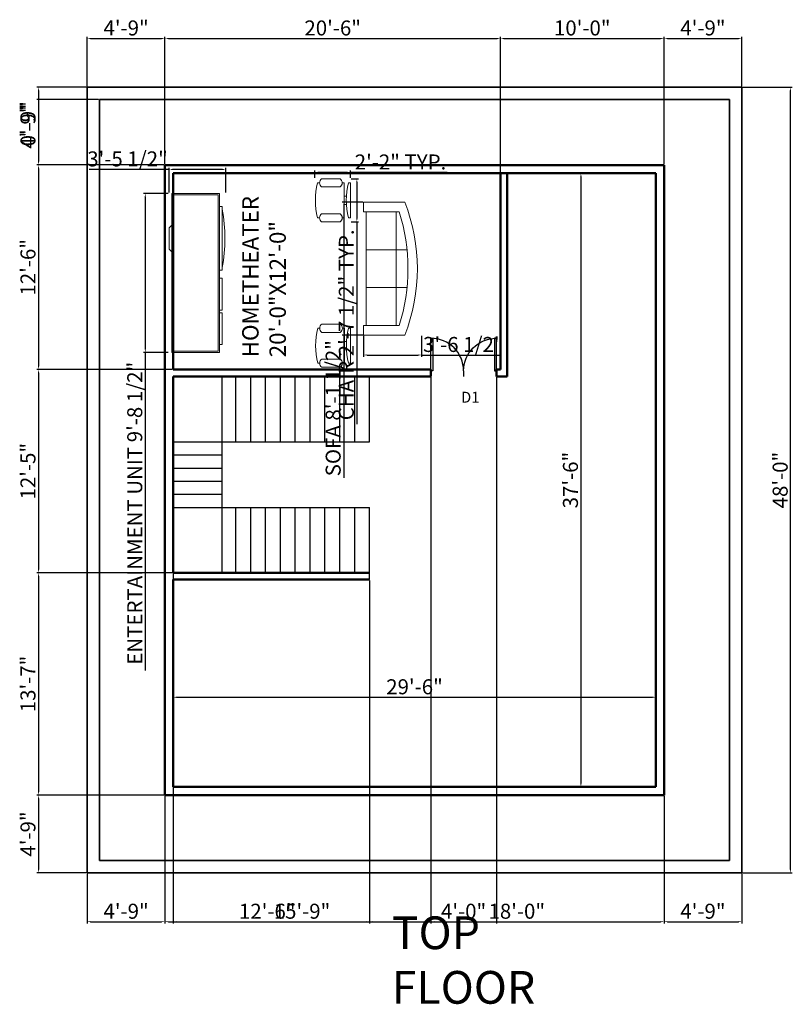
# Model space of a CAD drawing. Units: inches. Extents: x 2299 to 4423, y 1066 to 1805.
# Tile 7 of 7: x 3856 to 4423, y 1075 to 1796. Entities that reach past the tile are written whole.
import ezdxf

# ---------------------------------------------------------------- set-up
doc = ezdxf.new("R2010")
doc.units = ezdxf.units.IN
for name, color, linetype, lineweight in [('A-ANNO-DIMS', 2, 'Continuous', 18), ('A-ANNO-TEXT', 1, 'Continuous', 25), ('A-AREA-IDEN', 1, 'Continuous', 25), ('A-DOOR', 5, 'Continuous', 25), ('A-FLOR-STRS', 6, 'Continuous', 25), ('A-FURN', 8, 'Continuous', 18), ('A-WALL', 7, 'Continuous', 50), ('C-PROP', 7, 'Continuous', 35)]:
    doc.layers.add(name, color=color, linetype=linetype, lineweight=lineweight)
doc.styles.get("Standard").update_dxf_attribs({"font": 'arial.ttf'})
doc.dimstyles.new('ISO-25', dxfattribs={"dimtxt": 11, "dimasz": 2.5, "dimexe": 1.25, "dimexo": 0.625, "dimtad": 1, "dimlunit": 4, "dimtxsty": 'Standard', "dimcen": 2.5, "dimadec": 0, "dimazin": 0, "dimtfac": 1, "dimtmove": 0, "dimatfit": 3, "dimfxl": 1, "dimarcsym": 0})

# ---------------------------------------------------------------- blocks, each defined once
blk = doc.blocks.new('*U2')
for p, q in [((0, 0), (0, -5)), ((30, 0), (30, -5))]:
    blk.add_line(p, q)
blk.add_lwpolyline([(0, 0), (0, 30), (1.75, 30), (1.75, 0)], close=True)
blk.add_arc((0, 0), 30, 0, 90)
blk = doc.blocks.new('Entertainment Center')
for p, q in [((-4, 0), (-5, -1)), ((4, 0), (-4, 0)), ((5, -1), (4, 0)), ((-17, -19), (-17, -1)), ((-17, -1), (43, -1)), ((-16.5, -18.5), (-16.5, -1.5)), ((-16.5, -1.5), (42.5, -1.5)), ((42.5, -1.5), (42.5, -18.5)), ((43, -1), (43, -19)), ((42.5, -18.5), (-16.5, -18.5)), ((43, -19), (-17, -19)), ((-12, -20), (-12, -19)), ((12, -20), (-12, -20)), ((12, -19), (12, -20)), ((15, -20), (15, -19)), ((27, -20), (15, -20)), ((27, -19), (27, -20)), ((28, -20), (28, -19)), ((40, -20), (28, -20)), ((40, -19), (40, -20))]:
    blk.add_line(p, q)
blk.add_arc((0, 40), 61, 259.6111, 280.3889)
blk = doc.blocks.new('Sofa - Roundback 7 ft.')
for p, q in [((-36.000027, -34), (-36.000027, -11.4696)), ((-12.00002, -32.4421), (-12.00003, -6.5971)), ((11.99997, -32.4421), (11.99998, -6.5971)), ((35.99998, -34), (35.99998, -11.4696)), ((-35.999844, -13.3819), (35.9998, -13.3819)), ((-36.000027, -32.4421), (35.99998, -32.4421))]:
    blk.add_line(p, q)
for points in [[(-36.000027, -34), (-42.000027, -34), (-42.000027, -8)], [(41.99998, -8), (41.99998, -34), (35.99998, -34)]]:
    blk.add_lwpolyline(points)
for centre, radius, start, end in [((0, -114.25), 114.25, 68.43141, 111.5686), ((-0.00001, -127.1968), 121.1968, 72.72033, 107.2797)]:
    blk.add_arc(centre, radius, start, end)
blk = doc.blocks.new('Chair - Desk')
for p, q in [((-8.5, 0), (-8.5, -1)), ((-8.5, 0), (8.5, 0)), ((8.5, 0), (8.5, -1)), ((-8.5, -3), (-8.5, -4)), ((-8.5, -3), (8.5, -3)), ((-2, -3), (-2, -1.9355)), ((2, -1.9576), (2, -3)), ((8.5, -3), (8.5, -4)), ((-10.5, -5), (-10.5, -14)), ((-6.5, -14), (-6.5, -5)), ((6.5, -5), (6.5, -14)), ((10.5, -14), (10.5, -5)), ((-8.5, -15), (-8.5, -16)), ((8.5, -15), (8.5, -16))]:
    blk.add_line(p, q)
for centre, radius, start, end in [((-8.5, -6.5), 2.5, 36.8699, 143.1301), ((0, 34.625), 36.625, 256.5803, 283.4197), ((8.5, -6.5), 2.5, 36.8699, 143.1301), ((-8.5, -12.5), 2.5, 216.8699, 323.1301), ((8.5, -12.5), 2.5, 216.8699, 323.1301), ((0, 19.625), 36.625, 256.5803, 283.4197)]:
    blk.add_arc(centre, radius, start, end)
blk = doc.blocks.new('*D28')
at = {"layer": 'A-ANNO-DIMS', "color": 0, "lineweight": -2, "transparency": 16777216}
for p, q in [((3969.03, 1234.57), (3969.03, 1300.97)), ((3971.53, 1299.72), (4320.53, 1299.72)), ((4323.03, 1234.57), (4323.03, 1300.97))]:
    blk.add_line(p, q, dxfattribs=at)
at = {"layer": 'A-ANNO-DIMS', "color": 0, "transparency": 16777216}
for points in [[(3971.53, 1300.14), (3971.53, 1299.31), (3969.03, 1299.72)], [(4320.53, 1300.14), (4320.53, 1299.31), (4323.03, 1299.72)]]:
    blk.add_solid(points, dxfattribs=at)
at = {"layer": 'Defpoints', "color": 0, "transparency": 16777216}
for p in [(4323.03, 1299.72), (3969.03, 1233.95), (4323.03, 1233.95)]:
    blk.add_point(p, dxfattribs=at)
at = {"layer": 'A-ANNO-DIMS', "color": 0, "transparency": 16777216, "insert": (4146.03, 1305.96), "char_height": 11, "attachment_point": 5}
blk.add_mtext('29\'-6"', dxfattribs=at)
blk = doc.blocks.new('*D29')
at = {"layer": 'A-ANNO-DIMS', "color": 0, "lineweight": -2, "transparency": 16777216}
for p, q in [((4322.4, 1683.95), (4266.78, 1683.95)), ((4268.03, 1681.45), (4268.03, 1236.45)), ((4322.4, 1233.95), (4266.78, 1233.95))]:
    blk.add_line(p, q, dxfattribs=at)
at = {"layer": 'A-ANNO-DIMS', "color": 0, "transparency": 16777216}
for points in [[(4267.62, 1681.45), (4268.45, 1681.45), (4268.03, 1683.95)], [(4267.62, 1236.45), (4268.45, 1236.45), (4268.03, 1233.95)]]:
    blk.add_solid(points, dxfattribs=at)
at = {"layer": 'Defpoints', "color": 0, "transparency": 16777216}
for p in [(4323.03, 1683.95), (4268.03, 1233.95), (4323.03, 1233.95)]:
    blk.add_point(p, dxfattribs=at)
at = {"layer": 'A-ANNO-DIMS', "color": 0, "transparency": 16777216, "insert": (4261.79, 1458.95), "char_height": 11, "attachment_point": 5, "rotation": 90}
blk.add_mtext('37\'-6"', dxfattribs=at)
blk = doc.blocks.new('*D36')
at = {"layer": 'A-ANNO-DIMS', "color": 0, "lineweight": -2, "transparency": 16777216}
for p, q in [((4099.63, 1679.84), (4105, 1679.84)), ((4103.75, 1677.34), (4103.75, 1650.71)), ((4099.63, 1648.21), (4105, 1648.21)), ((4103.75, 1648.21), (4103.75, 1499.82))]:
    blk.add_line(p, q, dxfattribs=at)
at = {"layer": 'A-ANNO-DIMS', "color": 0, "transparency": 16777216}
for points in [[(4103.33, 1677.34), (4104.16, 1677.34), (4103.75, 1679.84)], [(4103.33, 1650.71), (4104.16, 1650.71), (4103.75, 1648.21)]]:
    blk.add_solid(points, dxfattribs=at)
at = {"layer": 'Defpoints', "color": 0, "transparency": 16777216}
for p in [(4099, 1679.84), (4099, 1648.21), (4103.75, 1648.21)]:
    blk.add_point(p, dxfattribs=at)
at = {"layer": 'A-ANNO-DIMS', "color": 0, "transparency": 16777216, "insert": (4097.44, 1572.76), "char_height": 11, "attachment_point": 5, "rotation": 90}
blk.add_mtext('CHAIR 2\'-7 1/2" TYP.', dxfattribs=at)
blk = doc.blocks.new('*D37')
at = {"layer": 'A-ANNO-DIMS', "color": 0, "lineweight": -2, "transparency": 16777216}
for p, q in [((4072.89, 1680.47), (4072.89, 1685.84)), ((4075.39, 1684.59), (4096.5, 1684.59)), ((4099, 1680.47), (4099, 1685.84)), ((4099, 1684.59), (4169.99, 1684.59))]:
    blk.add_line(p, q, dxfattribs=at)
at = {"layer": 'A-ANNO-DIMS', "color": 0, "transparency": 16777216}
for points in [[(4075.39, 1685), (4075.39, 1684.17), (4072.89, 1684.59)], [(4096.5, 1685), (4096.5, 1684.17), (4099, 1684.59)]]:
    blk.add_solid(points, dxfattribs=at)
at = {"layer": 'Defpoints', "color": 0, "transparency": 16777216}
for p in [(4099, 1684.59), (4072.89, 1679.84), (4099, 1679.84)]:
    blk.add_point(p, dxfattribs=at)
at = {"layer": 'A-ANNO-DIMS', "color": 0, "transparency": 16777216, "insert": (4135.75, 1690.74), "char_height": 11, "attachment_point": 5}
blk.add_mtext('2\'-2" TYP.', dxfattribs=at)
blk = doc.blocks.new('*D42')
at = {"layer": 'A-ANNO-DIMS', "color": 0, "lineweight": -2, "transparency": 16777216}
for p, q in [((3965.48, 1669.16), (3947.35, 1669.16)), ((3948.6, 1666.66), (3948.6, 1554.92)), ((3965.48, 1552.42), (3947.35, 1552.42)), ((3948.6, 1552.42), (3948.6, 1319.37))]:
    blk.add_line(p, q, dxfattribs=at)
at = {"layer": 'A-ANNO-DIMS', "color": 0, "transparency": 16777216}
for points in [[(3948.18, 1666.66), (3949.01, 1666.66), (3948.6, 1669.16)], [(3948.18, 1554.92), (3949.01, 1554.92), (3948.6, 1552.42)]]:
    blk.add_solid(points, dxfattribs=at)
at = {"layer": 'Defpoints', "color": 0, "transparency": 16777216}
for p in [(3966.11, 1669.16), (3948.6, 1552.42), (3966.11, 1552.42)]:
    blk.add_point(p, dxfattribs=at)
at = {"layer": 'A-ANNO-DIMS', "color": 0, "transparency": 16777216, "insert": (3942.29, 1434.64), "char_height": 11, "attachment_point": 5, "rotation": 90}
blk.add_mtext('ENTERTAINMENT UNIT 9\'-8 1/2"', dxfattribs=at)
blk = doc.blocks.new('*D43')
at = {"layer": 'A-ANNO-DIMS', "color": 0, "lineweight": -2, "transparency": 16777216}
for p, q in [((3966.11, 1686.67), (3907.49, 1686.67)), ((3966.11, 1669.79), (3966.11, 1687.92)), ((4005.12, 1686.67), (3968.61, 1686.67)), ((4007.62, 1669.79), (4007.62, 1687.92))]:
    blk.add_line(p, q, dxfattribs=at)
at = {"layer": 'A-ANNO-DIMS', "color": 0, "transparency": 16777216}
for points in [[(3968.61, 1687.09), (3968.61, 1686.25), (3966.11, 1686.67)], [(4005.12, 1687.09), (4005.12, 1686.25), (4007.62, 1686.67)]]:
    blk.add_solid(points, dxfattribs=at)
at = {"layer": 'Defpoints', "color": 0, "transparency": 16777216}
for p in [(3966.11, 1686.67), (3966.11, 1669.16), (4007.62, 1669.16)]:
    blk.add_point(p, dxfattribs=at)
at = {"layer": 'A-ANNO-DIMS', "color": 0, "transparency": 16777216, "insert": (3935.55, 1692.99), "char_height": 11, "attachment_point": 5}
blk.add_mtext('3\'-5 1/2"', dxfattribs=at)
blk = doc.blocks.new('*D54')
at = {"layer": 'A-ANNO-DIMS', "color": 0, "lineweight": -2, "transparency": 16777216}
for p, q in [((4108.1, 1662.66), (4092.86, 1662.66)), ((4094.11, 1660.16), (4094.11, 1567.74)), ((4108.1, 1565.24), (4092.86, 1565.24)), ((4094.11, 1565.24), (4094.11, 1460.56))]:
    blk.add_line(p, q, dxfattribs=at)
at = {"layer": 'A-ANNO-DIMS', "color": 0, "transparency": 16777216}
for points in [[(4093.7, 1660.16), (4094.53, 1660.16), (4094.11, 1662.66)], [(4093.7, 1567.74), (4094.53, 1567.74), (4094.11, 1565.24)]]:
    blk.add_solid(points, dxfattribs=at)
at = {"layer": 'Defpoints', "color": 0, "transparency": 16777216}
for p in [(4108.73, 1662.66), (4094.11, 1565.24), (4108.73, 1565.24)]:
    blk.add_point(p, dxfattribs=at)
at = {"layer": 'A-ANNO-DIMS', "color": 0, "transparency": 16777216, "insert": (4087.8, 1511.65), "char_height": 11, "attachment_point": 5, "rotation": 90}
blk.add_mtext('SOFA 8\'-1 1/2"', dxfattribs=at)
blk = doc.blocks.new('*D55')
at = {"layer": 'A-ANNO-DIMS', "color": 0, "lineweight": -2, "transparency": 16777216}
for p, q in [((4108.73, 1564.61), (4108.73, 1549.38)), ((4151.25, 1564.61), (4151.25, 1549.38)), ((4111.23, 1550.63), (4148.75, 1550.63)), ((4151.25, 1550.63), (4209.87, 1550.63))]:
    blk.add_line(p, q, dxfattribs=at)
at = {"layer": 'A-ANNO-DIMS', "color": 0, "transparency": 16777216}
for points in [[(4111.23, 1551.04), (4111.23, 1550.21), (4108.73, 1550.63)], [(4148.75, 1551.04), (4148.75, 1550.21), (4151.25, 1550.63)]]:
    blk.add_solid(points, dxfattribs=at)
at = {"layer": 'Defpoints', "color": 0, "transparency": 16777216}
for p in [(4108.73, 1565.24), (4151.25, 1565.24), (4151.25, 1550.63)]:
    blk.add_point(p, dxfattribs=at)
at = {"layer": 'A-ANNO-DIMS', "color": 0, "transparency": 16777216, "insert": (4181.81, 1556.94), "char_height": 11, "attachment_point": 5}
blk.add_mtext('3\'-6 1/2"', dxfattribs=at)
blk = doc.blocks.new('*D115')
at = {"layer": 'A-ANNO-DIMS', "color": 0, "lineweight": -2, "transparency": 16777216}
for p, q in [((3906.03, 1747.57), (3906.03, 1784)), ((3963.03, 1690.57), (3963.03, 1784)), ((3908.53, 1782.75), (3960.53, 1782.75))]:
    blk.add_line(p, q, dxfattribs=at)
at = {"layer": 'A-ANNO-DIMS', "color": 0, "transparency": 16777216}
for points in [[(3908.53, 1783.16), (3908.53, 1782.33), (3906.03, 1782.75)], [(3960.53, 1783.16), (3960.53, 1782.33), (3963.03, 1782.75)]]:
    blk.add_solid(points, dxfattribs=at)
at = {"layer": 'Defpoints', "color": 0, "transparency": 16777216}
for p in [(3963.03, 1782.75), (3906.03, 1746.95), (3963.03, 1689.95)]:
    blk.add_point(p, dxfattribs=at)
at = {"layer": 'A-ANNO-DIMS', "color": 0, "transparency": 16777216, "insert": (3934.53, 1788.99), "char_height": 11, "attachment_point": 5}
blk.add_mtext('4\'-9"', dxfattribs=at)
blk = doc.blocks.new('*D116')
at = {"layer": 'A-ANNO-DIMS', "color": 0, "lineweight": -2, "transparency": 16777216}
for p, q in [((3963.03, 1690.57), (3963.03, 1784)), ((4209.03, 1684.57), (4209.03, 1784)), ((3965.53, 1782.75), (4206.53, 1782.75))]:
    blk.add_line(p, q, dxfattribs=at)
at = {"layer": 'A-ANNO-DIMS', "color": 0, "transparency": 16777216}
for points in [[(3965.53, 1783.16), (3965.53, 1782.33), (3963.03, 1782.75)], [(4206.53, 1783.16), (4206.53, 1782.33), (4209.03, 1782.75)]]:
    blk.add_solid(points, dxfattribs=at)
at = {"layer": 'Defpoints', "color": 0, "transparency": 16777216}
for p in [(4209.03, 1782.75), (3963.03, 1689.95), (4209.03, 1683.95)]:
    blk.add_point(p, dxfattribs=at)
at = {"layer": 'A-ANNO-DIMS', "color": 0, "transparency": 16777216, "insert": (4086.03, 1788.99), "char_height": 11, "attachment_point": 5}
blk.add_mtext('20\'-6"', dxfattribs=at)
blk = doc.blocks.new('*D117')
at = {"layer": 'A-ANNO-DIMS', "color": 0, "lineweight": -2, "transparency": 16777216}
for p, q in [((4209.03, 1684.57), (4209.03, 1784)), ((4329.03, 1690.57), (4329.03, 1784)), ((4211.53, 1782.75), (4326.53, 1782.75))]:
    blk.add_line(p, q, dxfattribs=at)
at = {"layer": 'A-ANNO-DIMS', "color": 0, "transparency": 16777216}
for points in [[(4211.53, 1783.16), (4211.53, 1782.33), (4209.03, 1782.75)], [(4326.53, 1783.16), (4326.53, 1782.33), (4329.03, 1782.75)]]:
    blk.add_solid(points, dxfattribs=at)
at = {"layer": 'Defpoints', "color": 0, "transparency": 16777216}
for p in [(4329.03, 1782.75), (4329.03, 1689.95), (4209.03, 1683.95)]:
    blk.add_point(p, dxfattribs=at)
at = {"layer": 'A-ANNO-DIMS', "color": 0, "transparency": 16777216, "insert": (4269.03, 1788.99), "char_height": 11, "attachment_point": 5}
blk.add_mtext('10\'-0"', dxfattribs=at)
blk = doc.blocks.new('*D118')
at = {"layer": 'A-ANNO-DIMS', "color": 0, "lineweight": -2, "transparency": 16777216}
for p, q in [((4329.03, 1690.57), (4329.03, 1784)), ((4386.03, 1747.57), (4386.03, 1784)), ((4331.53, 1782.75), (4383.53, 1782.75))]:
    blk.add_line(p, q, dxfattribs=at)
at = {"layer": 'A-ANNO-DIMS', "color": 0, "transparency": 16777216}
for points in [[(4331.53, 1783.16), (4331.53, 1782.33), (4329.03, 1782.75)], [(4383.53, 1783.16), (4383.53, 1782.33), (4386.03, 1782.75)]]:
    blk.add_solid(points, dxfattribs=at)
at = {"layer": 'Defpoints', "color": 0, "transparency": 16777216}
for p in [(4386.03, 1782.75), (4386.03, 1746.95), (4329.03, 1689.95)]:
    blk.add_point(p, dxfattribs=at)
at = {"layer": 'A-ANNO-DIMS', "color": 0, "transparency": 16777216, "insert": (4357.53, 1788.99), "char_height": 11, "attachment_point": 5}
blk.add_mtext('4\'-9"', dxfattribs=at)
blk = doc.blocks.new('*D119')
at = {"layer": 'A-ANNO-DIMS', "color": 0, "lineweight": -2, "transparency": 16777216}
for p, q in [((3905.4, 1746.95), (3868.98, 1746.95)), ((3870.23, 1744.45), (3870.23, 1692.45)), ((3962.4, 1689.95), (3868.98, 1689.95))]:
    blk.add_line(p, q, dxfattribs=at)
at = {"layer": 'A-ANNO-DIMS', "color": 0, "transparency": 16777216}
for points in [[(3869.81, 1744.45), (3870.64, 1744.45), (3870.23, 1746.95)], [(3869.81, 1692.45), (3870.64, 1692.45), (3870.23, 1689.95)]]:
    blk.add_solid(points, dxfattribs=at)
at = {"layer": 'Defpoints', "color": 0, "transparency": 16777216}
for p in [(3906.03, 1746.95), (3870.23, 1689.95), (3963.03, 1689.95)]:
    blk.add_point(p, dxfattribs=at)
at = {"layer": 'A-ANNO-DIMS', "color": 0, "transparency": 16777216, "insert": (3863.99, 1718.45), "char_height": 11, "attachment_point": 5, "rotation": 90}
blk.add_mtext('4\'-9"', dxfattribs=at)
blk = doc.blocks.new('*D120')
at = {"layer": 'A-ANNO-DIMS', "color": 0, "lineweight": -2, "transparency": 16777216}
for p, q in [((3962.4, 1689.95), (3868.98, 1689.95)), ((3870.23, 1687.45), (3870.23, 1542.45)), ((3968.4, 1539.95), (3868.98, 1539.95))]:
    blk.add_line(p, q, dxfattribs=at)
at = {"layer": 'A-ANNO-DIMS', "color": 0, "transparency": 16777216}
for points in [[(3869.81, 1687.45), (3870.64, 1687.45), (3870.23, 1689.95)], [(3869.81, 1542.45), (3870.64, 1542.45), (3870.23, 1539.95)]]:
    blk.add_solid(points, dxfattribs=at)
at = {"layer": 'Defpoints', "color": 0, "transparency": 16777216}
for p in [(3963.03, 1689.95), (3870.23, 1539.95), (3969.03, 1539.95)]:
    blk.add_point(p, dxfattribs=at)
at = {"layer": 'A-ANNO-DIMS', "color": 0, "transparency": 16777216, "insert": (3863.99, 1614.95), "char_height": 11, "attachment_point": 5, "rotation": 90}
blk.add_mtext('12\'-6"', dxfattribs=at)
blk = doc.blocks.new('*D121')
at = {"layer": 'A-ANNO-DIMS', "color": 0, "lineweight": -2, "transparency": 16777216}
for p, q in [((3968.4, 1539.95), (3868.98, 1539.95)), ((3870.23, 1537.45), (3870.23, 1393.45)), ((3968.4, 1390.95), (3868.98, 1390.95))]:
    blk.add_line(p, q, dxfattribs=at)
at = {"layer": 'A-ANNO-DIMS', "color": 0, "transparency": 16777216}
for points in [[(3869.81, 1537.45), (3870.64, 1537.45), (3870.23, 1539.95)], [(3869.81, 1393.45), (3870.64, 1393.45), (3870.23, 1390.95)]]:
    blk.add_solid(points, dxfattribs=at)
at = {"layer": 'Defpoints', "color": 0, "transparency": 16777216}
for p in [(3969.03, 1539.95), (3870.23, 1390.95), (3969.03, 1390.95)]:
    blk.add_point(p, dxfattribs=at)
at = {"layer": 'A-ANNO-DIMS', "color": 0, "transparency": 16777216, "insert": (3863.99, 1465.45), "char_height": 11, "attachment_point": 5, "rotation": 90}
blk.add_mtext('12\'-5"', dxfattribs=at)
blk = doc.blocks.new('*D122')
at = {"layer": 'A-ANNO-DIMS', "color": 0, "lineweight": -2, "transparency": 16777216}
for p, q in [((3968.4, 1390.95), (3868.98, 1390.95)), ((3870.23, 1388.45), (3870.23, 1230.45)), ((3962.4, 1227.95), (3868.98, 1227.95))]:
    blk.add_line(p, q, dxfattribs=at)
at = {"layer": 'A-ANNO-DIMS', "color": 0, "transparency": 16777216}
for points in [[(3869.81, 1388.45), (3870.64, 1388.45), (3870.23, 1390.95)], [(3869.81, 1230.45), (3870.64, 1230.45), (3870.23, 1227.95)]]:
    blk.add_solid(points, dxfattribs=at)
at = {"layer": 'Defpoints', "color": 0, "transparency": 16777216}
for p in [(3969.03, 1390.95), (3870.23, 1227.95), (3963.03, 1227.95)]:
    blk.add_point(p, dxfattribs=at)
at = {"layer": 'A-ANNO-DIMS', "color": 0, "transparency": 16777216, "insert": (3863.98, 1309.45), "char_height": 11, "attachment_point": 5, "rotation": 90}
blk.add_mtext('13\'-7"', dxfattribs=at)
blk = doc.blocks.new('*D123')
at = {"layer": 'A-ANNO-DIMS', "color": 0, "lineweight": -2, "transparency": 16777216}
for p, q in [((3962.4, 1227.95), (3868.98, 1227.95)), ((3870.23, 1225.45), (3870.23, 1173.45)), ((3905.4, 1170.95), (3868.98, 1170.95))]:
    blk.add_line(p, q, dxfattribs=at)
at = {"layer": 'A-ANNO-DIMS', "color": 0, "transparency": 16777216}
for points in [[(3869.81, 1225.45), (3870.64, 1225.45), (3870.23, 1227.95)], [(3869.81, 1173.45), (3870.64, 1173.45), (3870.23, 1170.95)]]:
    blk.add_solid(points, dxfattribs=at)
at = {"layer": 'Defpoints', "color": 0, "transparency": 16777216}
for p in [(3963.03, 1227.95), (3870.23, 1170.95), (3906.03, 1170.95)]:
    blk.add_point(p, dxfattribs=at)
at = {"layer": 'A-ANNO-DIMS', "color": 0, "transparency": 16777216, "insert": (3863.99, 1199.45), "char_height": 11, "attachment_point": 5, "rotation": 90}
blk.add_mtext('4\'-9"', dxfattribs=at)
blk = doc.blocks.new('*D124')
at = {"layer": 'A-ANNO-DIMS', "color": 0, "lineweight": -2, "transparency": 16777216}
for p, q in [((3905.4, 1746.95), (3868.98, 1746.95)), ((3870.23, 1744.45), (3870.23, 1740.45)), ((3914.4, 1737.95), (3868.98, 1737.95)), ((3870.23, 1737.95), (3870.23, 1704.95))]:
    blk.add_line(p, q, dxfattribs=at)
at = {"layer": 'A-ANNO-DIMS', "color": 0, "transparency": 16777216}
for points in [[(3869.81, 1744.45), (3870.64, 1744.45), (3870.23, 1746.95)], [(3869.81, 1740.45), (3870.64, 1740.45), (3870.23, 1737.95)]]:
    blk.add_solid(points, dxfattribs=at)
at = {"layer": 'Defpoints', "color": 0, "transparency": 16777216}
for p in [(3906.03, 1746.95), (3870.23, 1737.95), (3915.03, 1737.95)]:
    blk.add_point(p, dxfattribs=at)
at = {"layer": 'A-ANNO-DIMS', "color": 0, "transparency": 16777216, "insert": (3863.99, 1720.2), "char_height": 11, "attachment_point": 5, "rotation": 90}
blk.add_mtext('0\'-9"', dxfattribs=at)
blk = doc.blocks.new('*D125')
at = {"layer": 'A-ANNO-DIMS', "color": 0, "lineweight": -2, "transparency": 16777216}
for p, q in [((4386.65, 1746.95), (4423.08, 1746.95)), ((4421.83, 1173.45), (4421.83, 1744.45)), ((4386.65, 1170.95), (4423.08, 1170.95))]:
    blk.add_line(p, q, dxfattribs=at)
at = {"layer": 'A-ANNO-DIMS', "color": 0, "transparency": 16777216}
for points in [[(4421.41, 1744.45), (4422.24, 1744.45), (4421.83, 1746.95)], [(4421.41, 1173.45), (4422.24, 1173.45), (4421.83, 1170.95)]]:
    blk.add_solid(points, dxfattribs=at)
at = {"layer": 'Defpoints', "color": 0, "transparency": 16777216}
for p in [(4386.03, 1746.95), (4421.83, 1746.95), (4386.03, 1170.95)]:
    blk.add_point(p, dxfattribs=at)
at = {"layer": 'A-ANNO-DIMS', "color": 0, "transparency": 16777216, "insert": (4415.59, 1458.95), "char_height": 11, "attachment_point": 5, "rotation": 90}
blk.add_mtext('48\'-0"', dxfattribs=at)
blk = doc.blocks.new('*D126')
at = {"layer": 'A-ANNO-DIMS', "color": 0, "lineweight": -2, "transparency": 16777216}
for p, q in [((3963.03, 1227.32), (3963.03, 1133.9)), ((3906.03, 1170.32), (3906.03, 1133.9)), ((3908.53, 1135.15), (3960.53, 1135.15))]:
    blk.add_line(p, q, dxfattribs=at)
at = {"layer": 'A-ANNO-DIMS', "color": 0, "transparency": 16777216}
for points in [[(3908.53, 1135.56), (3908.53, 1134.73), (3906.03, 1135.15)], [(3960.53, 1135.56), (3960.53, 1134.73), (3963.03, 1135.15)]]:
    blk.add_solid(points, dxfattribs=at)
at = {"layer": 'Defpoints', "color": 0, "transparency": 16777216}
for p in [(3963.03, 1227.95), (3906.03, 1170.95), (3963.03, 1135.15)]:
    blk.add_point(p, dxfattribs=at)
at = {"layer": 'A-ANNO-DIMS', "color": 0, "transparency": 16777216, "insert": (3934.53, 1141.39), "char_height": 11, "attachment_point": 5}
blk.add_mtext('4\'-9"', dxfattribs=at)
blk = doc.blocks.new('*D127')
at = {"layer": 'A-ANNO-DIMS', "color": 0, "lineweight": -2, "transparency": 16777216}
for p, q in [((4113.03, 1385.32), (4113.03, 1133.9)), ((3963.03, 1227.32), (3963.03, 1133.9)), ((3965.53, 1135.15), (4110.53, 1135.15))]:
    blk.add_line(p, q, dxfattribs=at)
at = {"layer": 'A-ANNO-DIMS', "color": 0, "transparency": 16777216}
for points in [[(3965.53, 1135.56), (3965.53, 1134.73), (3963.03, 1135.15)], [(4110.53, 1135.56), (4110.53, 1134.73), (4113.03, 1135.15)]]:
    blk.add_solid(points, dxfattribs=at)
at = {"layer": 'Defpoints', "color": 0, "transparency": 16777216}
for p in [(4113.03, 1385.95), (3963.03, 1227.95), (4113.03, 1135.15)]:
    blk.add_point(p, dxfattribs=at)
at = {"layer": 'A-ANNO-DIMS', "color": 0, "transparency": 16777216, "insert": (4038.03, 1141.39), "char_height": 11, "attachment_point": 5}
blk.add_mtext('12\'-6"', dxfattribs=at)
blk = doc.blocks.new('*D128')
at = {"layer": 'A-ANNO-DIMS', "color": 0, "lineweight": -2, "transparency": 16777216}
for p, q in [((4113.03, 1385.32), (4113.03, 1133.9)), ((4329.03, 1227.32), (4329.03, 1133.9)), ((4115.53, 1135.15), (4326.53, 1135.15))]:
    blk.add_line(p, q, dxfattribs=at)
at = {"layer": 'A-ANNO-DIMS', "color": 0, "transparency": 16777216}
for points in [[(4115.53, 1135.56), (4115.53, 1134.73), (4113.03, 1135.15)], [(4326.53, 1135.56), (4326.53, 1134.73), (4329.03, 1135.15)]]:
    blk.add_solid(points, dxfattribs=at)
at = {"layer": 'Defpoints', "color": 0, "transparency": 16777216}
for p in [(4113.03, 1385.95), (4329.03, 1227.95), (4329.03, 1135.15)]:
    blk.add_point(p, dxfattribs=at)
at = {"layer": 'A-ANNO-DIMS', "color": 0, "transparency": 16777216, "insert": (4221.03, 1141.39), "char_height": 11, "attachment_point": 5}
blk.add_mtext('18\'-0"', dxfattribs=at)
blk = doc.blocks.new('*D129')
at = {"layer": 'A-ANNO-DIMS', "color": 0, "lineweight": -2, "transparency": 16777216}
for p, q in [((4329.03, 1227.32), (4329.03, 1133.9)), ((4386.03, 1170.32), (4386.03, 1133.9)), ((4331.53, 1135.15), (4383.53, 1135.15))]:
    blk.add_line(p, q, dxfattribs=at)
at = {"layer": 'A-ANNO-DIMS', "color": 0, "transparency": 16777216}
for points in [[(4331.53, 1135.56), (4331.53, 1134.73), (4329.03, 1135.15)], [(4383.53, 1135.56), (4383.53, 1134.73), (4386.03, 1135.15)]]:
    blk.add_solid(points, dxfattribs=at)
at = {"layer": 'Defpoints', "color": 0, "transparency": 16777216}
for p in [(4329.03, 1227.95), (4386.03, 1170.95), (4386.03, 1135.15)]:
    blk.add_point(p, dxfattribs=at)
at = {"layer": 'A-ANNO-DIMS', "color": 0, "transparency": 16777216, "insert": (4357.53, 1141.39), "char_height": 11, "attachment_point": 5}
blk.add_mtext('4\'-9"', dxfattribs=at)
blk = doc.blocks.new('*D130')
at = {"layer": 'A-ANNO-DIMS', "color": 0, "lineweight": -2, "transparency": 16777216}
for p, q in [((3969.03, 1534.32), (3969.03, 1133.9)), ((4158.03, 1534.32), (4158.03, 1133.9)), ((3971.53, 1135.15), (4155.53, 1135.15))]:
    blk.add_line(p, q, dxfattribs=at)
at = {"layer": 'A-ANNO-DIMS', "color": 0, "transparency": 16777216}
for points in [[(3971.53, 1135.56), (3971.53, 1134.73), (3969.03, 1135.15)], [(4155.53, 1135.56), (4155.53, 1134.73), (4158.03, 1135.15)]]:
    blk.add_solid(points, dxfattribs=at)
at = {"layer": 'Defpoints', "color": 0, "transparency": 16777216}
for p in [(3969.03, 1534.95), (4158.03, 1534.95), (4158.03, 1135.15)]:
    blk.add_point(p, dxfattribs=at)
at = {"layer": 'A-ANNO-DIMS', "color": 0, "transparency": 16777216, "insert": (4063.53, 1141.39), "char_height": 11, "attachment_point": 5}
blk.add_mtext('15\'-9"', dxfattribs=at)
blk = doc.blocks.new('*D131')
at = {"layer": 'A-ANNO-DIMS', "color": 0, "lineweight": -2, "transparency": 16777216}
for p, q in [((4158.03, 1534.32), (4158.03, 1133.9)), ((4206.03, 1534.32), (4206.03, 1133.9)), ((4160.53, 1135.15), (4203.53, 1135.15))]:
    blk.add_line(p, q, dxfattribs=at)
at = {"layer": 'A-ANNO-DIMS', "color": 0, "transparency": 16777216}
for points in [[(4160.53, 1135.56), (4160.53, 1134.73), (4158.03, 1135.15)], [(4203.53, 1135.56), (4203.53, 1134.73), (4206.03, 1135.15)]]:
    blk.add_solid(points, dxfattribs=at)
at = {"layer": 'Defpoints', "color": 0, "transparency": 16777216}
for p in [(4158.03, 1534.95), (4206.03, 1534.95), (4206.03, 1135.15)]:
    blk.add_point(p, dxfattribs=at)
at = {"layer": 'A-ANNO-DIMS', "color": 0, "transparency": 16777216, "insert": (4182.03, 1141.39), "char_height": 11, "attachment_point": 5}
blk.add_mtext('4\'-0"', dxfattribs=at)

msp = doc.modelspace()

# ---------------------------------------------------------------- linework, layer by layer
at = {"layer": 'A-FLOR-STRS'}
for p, q in [((4005.027, 1534.945), (3969.027, 1534.945)), ((3969.027, 1534.945), (3969.027, 1390.945)), ((4005.027, 1390.945), (4005.027, 1534.945)), ((4015.027, 1486.945), (4015.027, 1534.945)), ((4025.916, 1486.945), (4025.916, 1534.945)), ((4036.805, 1486.945), (4036.805, 1534.945)), ((4047.694, 1486.945), (4047.694, 1534.945)), ((4058.583, 1486.945), (4058.583, 1534.945)), ((4069.472, 1486.945), (4069.472, 1534.945)), ((4080.361, 1486.945), (4080.361, 1534.945)), ((4091.25, 1486.945), (4091.25, 1534.945)), ((4102.139, 1486.945), (4102.139, 1534.945)), ((4113.027, 1486.945), (4113.027, 1534.945)), ((4113.027, 1486.945), (4113.027, 1534.945)), ((3969.027, 1486.945), (4113.027, 1486.945)), ((3969.027, 1477.345), (4005.027, 1477.345)), ((3969.027, 1467.745), (4005.027, 1467.745)), ((3969.027, 1458.145), (4005.027, 1458.145)), ((3969.027, 1448.545), (4005.027, 1448.545)), ((3969.027, 1438.945), (4113.027, 1438.945)), ((3969.027, 1438.945), (4113.027, 1438.945)), ((4015.027, 1390.945), (4015.027, 1438.945)), ((4025.916, 1390.945), (4025.916, 1438.945)), ((4036.805, 1390.945), (4036.805, 1438.945)), ((4047.694, 1390.945), (4047.694, 1438.945)), ((4058.583, 1390.945), (4058.583, 1438.945)), ((4069.472, 1390.945), (4069.472, 1438.945)), ((4080.361, 1390.945), (4080.361, 1438.945)), ((4091.25, 1390.945), (4091.25, 1438.945)), ((4102.139, 1390.945), (4102.139, 1438.945)), ((4113.027, 1390.945), (4113.027, 1438.945)), ((4113.027, 1385.945), (4113.027, 1438.945)), ((3969.027, 1390.945), (4005.027, 1390.945))]:
    msp.add_line(p, q, dxfattribs=at)
at = {"layer": 'A-WALL'}
for p, q in [((3963.027, 1227.945), (3963.027, 1689.945)), ((3963.027, 1689.945), (4329.027, 1689.945)), ((4329.027, 1689.945), (4329.027, 1486.945)), ((3969.027, 1539.945), (3969.027, 1683.945)), ((3969.027, 1683.945), (4113.027, 1683.945)), ((3969.027, 1683.945), (4323.027, 1683.945)), ((4183.027, 1683.945), (4323.027, 1683.945)), ((4209.027, 1539.945), (4209.027, 1683.945)), ((4214.027, 1534.945), (4214.027, 1683.945)), ((4323.027, 1683.945), (4323.027, 1539.945)), ((4323.027, 1683.945), (4323.027, 1486.945)), ((3969.027, 1539.945), (4113.027, 1539.945)), ((3969.027, 1539.945), (4158.027, 1539.945)), ((4158.027, 1539.945), (4158.027, 1534.945)), ((4206.027, 1539.945), (4209.027, 1539.945)), ((4206.027, 1539.945), (4209.027, 1539.945)), ((4206.027, 1539.945), (4206.027, 1534.945)), ((3969.027, 1390.945), (3969.027, 1534.945)), ((3969.027, 1534.945), (4158.027, 1534.945)), ((4206.027, 1534.945), (4214.027, 1534.945)), ((4323.027, 1486.945), (4323.027, 1233.945)), ((4329.027, 1486.945), (4329.027, 1227.945)), ((3969.027, 1390.945), (4113.027, 1390.945)), ((3969.027, 1233.945), (3969.027, 1385.945)), ((3969.027, 1385.945), (4113.027, 1385.945)), ((3963.027, 1227.945), (4329.027, 1227.945)), ((4323.027, 1233.945), (3969.027, 1233.945))]:
    msp.add_line(p, q, dxfattribs=at)
at = {"layer": 'C-PROP'}
for p, q in [((3906.027, 1170.945), (3906.027, 1746.945)), ((3906.027, 1746.945), (4386.027, 1746.945)), ((4386.027, 1746.945), (4386.027, 1170.945)), ((3915.027, 1179.945), (3915.027, 1737.945)), ((3915.027, 1737.945), (4377.027, 1737.945)), ((4377.027, 1737.945), (4377.027, 1179.945)), ((4377.027, 1179.945), (3915.027, 1179.945)), ((4386.027, 1170.945), (3906.027, 1170.945))]:
    msp.add_line(p, q, dxfattribs=at)

# ---------------------------------------------------------------- block references
at = {"layer": 'A-DOOR', "yscale": 0.7999999999999965, "zscale": 0.7999999999999965}
for p, xscale in [((4158.027, 1538.945), 0.7999999999999965), ((4206.027, 1538.945), -0.7999999999999965)]:
    msp.add_blockref('*U2', p, dxfattribs=dict(at, xscale=xscale))
at = {"layer": 'A-FURN'}
for name, p, xscale, yscale, zscale, rotation in [('Chair - Desk', (4099.003, 1664.024), 1.506486368633179, 1.506486368633179, 1.506486368633179, 270), ('Entertainment Center', (3966.109, 1636.084), -1.945664435241785, 1.945664435241785, 1.945664435241785, 90), ('Sofa - Roundback 7 ft.', (4148.16, 1613.95), 1.159768782470955, 1.159768782470955, 1.159768782470955, 270), ('Chair - Desk', (4099.132, 1557.442), 1.506486368633179, 1.506486368633179, 1.506486368633179, 270)]:
    msp.add_blockref(name, p, dxfattribs=dict(at, xscale=xscale, yscale=yscale, zscale=zscale, rotation=rotation))

# ---------------------------------------------------------------- texts
at = {"layer": 'A-ANNO-TEXT', "attachment_point": 1}
for s, width, gutter_width, insert, char_height in [('D1', 1.11117, 12.5, (4180.12, 1523.674), 8), ('TOP\\PFLOOR', 684.73543, 351.786, (4129.366, 1139.01), 24)]:
    msp.add_mtext_dynamic_manual_height_columns(s, width=width, gutter_width=gutter_width, heights=[0], dxfattribs=dict(at, insert=insert, char_height=char_height))
at = {"layer": 'A-AREA-IDEN', "insert": (4019.67, 1548.986), "char_height": 12, "attachment_point": 1, "rotation": 90}
msp.add_mtext_dynamic_manual_height_columns('HOMETHEATER\\P20\'-0"X12\'-0"', width=9.28623, gutter_width=12.5, heights=[0], dxfattribs=at)

# ---------------------------------------------------------------- dimensions: what is measured, and where the dimension line sits
at = {"layer": 'A-ANNO-DIMS'}
for base, p1, p2, override, picture, middle in [((3963.027, 1782.745), (3906.027, 1746.945), (3963.027, 1689.945), {"dimdec": 1, "dimlfac": 1, "dimrnd": 0, "dimzin": 1, "dimdsep": 46, "dimlunit": 4, "dimfrac": 2}, '*D115', (3934.527, 1788.987)), ((4209.027, 1782.745), (3963.027, 1689.945), (4209.027, 1683.945), {"dimdec": 1, "dimlfac": 1, "dimrnd": 0, "dimzin": 1, "dimdsep": 46, "dimlunit": 4, "dimfrac": 2}, '*D116', (4086.027, 1788.987)), ((4329.027, 1782.745), (4209.027, 1683.945), (4329.027, 1689.945), {"dimdec": 1, "dimlfac": 1, "dimrnd": 0, "dimzin": 1, "dimdsep": 46, "dimlunit": 4, "dimfrac": 2}, '*D117', (4269.027, 1788.987)), ((4386.027, 1782.745), (4329.027, 1689.945), (4386.027, 1746.945), {"dimdec": 1, "dimlfac": 1, "dimrnd": 0, "dimzin": 1, "dimdsep": 46, "dimlunit": 4, "dimfrac": 2}, '*D118', (4357.527, 1788.987)), ((4151.253, 1550.627), (4108.728, 1565.24), (4151.253, 1565.24), {"dimdec": 1, "dimrnd": 0, "dimzin": 1, "dimlunit": 4, "dimfrac": 2}, '*D55', (4181.81, 1556.943)), ((4158.027, 1135.145), (3969.027, 1534.945), (4158.027, 1534.945), {"dimdec": 1, "dimlfac": 1, "dimrnd": 0, "dimzin": 1, "dimdsep": 46, "dimlunit": 4, "dimfrac": 2}, '*D130', (4063.527, 1141.387)), ((4206.027, 1135.145), (4158.027, 1534.945), (4206.027, 1534.945), {"dimdec": 1, "dimlfac": 1, "dimrnd": 0, "dimzin": 1, "dimdsep": 46, "dimlunit": 4, "dimfrac": 2}, '*D131', (4182.027, 1141.387)), ((4113.027, 1135.145), (3963.027, 1227.945), (4113.027, 1385.945), {"dimdec": 1, "dimlfac": 1, "dimrnd": 0, "dimzin": 1, "dimdsep": 46, "dimlunit": 4, "dimfrac": 2}, '*D127', (4038.027, 1141.387)), ((4329.027, 1135.145), (4113.027, 1385.945), (4329.027, 1227.945), {"dimdec": 1, "dimlfac": 1, "dimrnd": 0, "dimzin": 1, "dimdsep": 46, "dimlunit": 4, "dimfrac": 2}, '*D128', (4221.027, 1141.387)), ((4323.027, 1299.723), (3969.027, 1233.945), (4323.027, 1233.945), {"dimclrd": 0, "dimclre": 0, "dimclrt": 0}, '*D28', (4146.027, 1305.964)), ((3963.027, 1135.145), (3906.027, 1170.945), (3963.027, 1227.945), {"dimdec": 1, "dimlfac": 1, "dimrnd": 0, "dimzin": 1, "dimdsep": 46, "dimlunit": 4, "dimfrac": 2}, '*D126', (3934.527, 1141.387)), ((4386.027, 1135.145), (4329.027, 1227.945), (4386.027, 1170.945), {"dimdec": 1, "dimlfac": 1, "dimrnd": 0, "dimzin": 1, "dimdsep": 46, "dimlunit": 4, "dimfrac": 2}, '*D129', (4357.527, 1141.387))]:
    dim = msp.add_linear_dim(base=base, p1=p1, p2=p2, dimstyle='ISO-25', override=override, dxfattribs=at)
    dim.commit()
    dim.dimension.update_dxf_attribs({"geometry": picture, "text_midpoint": middle})
for base, p1, p2, angle, override, picture, middle in [((3870.227, 1689.945), (3906.027, 1746.945), (3963.027, 1689.945), 90, {"dimdec": 1, "dimlfac": 1, "dimrnd": 0, "dimzin": 1, "dimdsep": 46, "dimlunit": 4, "dimfrac": 2}, '*D119', (3863.986, 1718.445)), ((3870.227, 1737.945), (3906.027, 1746.945), (3915.027, 1737.945), 90, {"dimdec": 1, "dimlfac": 1, "dimrnd": 0, "dimzin": 1, "dimdsep": 46, "dimlunit": 4, "dimfrac": 2}, '*D124', (3863.986, 1720.2)), ((4421.827, 1746.945), (4386.027, 1170.945), (4386.027, 1746.945), 90, {"dimdec": 1, "dimlfac": 1, "dimrnd": 0, "dimzin": 1, "dimdsep": 46, "dimlunit": 4, "dimfrac": 2}, '*D125', (4415.586, 1458.945)), ((3966.109, 1686.672), (4007.616, 1669.161), (3966.109, 1669.161), 180, {"dimdec": 1, "dimrnd": 0, "dimzin": 1, "dimlunit": 4, "dimfrac": 2}, '*D43', (3935.551, 1692.988)), ((3870.227, 1539.945), (3963.027, 1689.945), (3969.027, 1539.945), 90, {"dimdec": 1, "dimlfac": 1, "dimrnd": 0, "dimzin": 1, "dimdsep": 46, "dimlunit": 4, "dimfrac": 2}, '*D120', (3863.986, 1614.945)), ((4268.034, 1233.945), (4323.027, 1683.945), (4323.027, 1233.945), 90, {"dimclrd": 0, "dimclre": 0, "dimclrt": 0}, '*D29', (4261.789, 1458.945)), ((3870.227, 1390.945), (3969.027, 1539.945), (3969.027, 1390.945), 90, {"dimdec": 1, "dimlfac": 1, "dimrnd": 0, "dimzin": 1, "dimdsep": 46, "dimlunit": 4, "dimfrac": 2}, '*D121', (3863.986, 1465.445)), ((3870.227, 1227.945), (3969.027, 1390.945), (3963.027, 1227.945), 90, {"dimdec": 1, "dimlfac": 1, "dimrnd": 0, "dimzin": 1, "dimdsep": 46, "dimlunit": 4, "dimfrac": 2}, '*D122', (3863.982, 1309.445)), ((3870.227, 1170.945), (3963.027, 1227.945), (3906.027, 1170.945), 90, {"dimdec": 1, "dimlfac": 1, "dimrnd": 0, "dimzin": 1, "dimdsep": 46, "dimlunit": 4, "dimfrac": 2}, '*D123', (3863.986, 1199.445))]:
    dim = msp.add_linear_dim(base=base, p1=p1, p2=p2, angle=angle, dimstyle='ISO-25', override=override, dxfattribs=at)
    dim.commit()
    dim.dimension.update_dxf_attribs({"geometry": picture, "text_midpoint": middle})
dim = msp.add_linear_dim(base=(4099.003, 1684.588), p1=(4072.89, 1679.843), p2=(4099.003, 1679.843), text='<> TYP.', dimstyle='ISO-25', override={"dimdec": 1, "dimrnd": 0, "dimzin": 1, "dimlunit": 4, "dimfrac": 2}, dxfattribs=at)
dim.commit()
dim.dimension.update_dxf_attribs({"geometry": '*D37', "text_midpoint": (4135.747, 1690.739)})
for base, p1, p2, text, picture, middle in [((4103.748, 1648.206), (4099.003, 1679.843), (4099.003, 1648.206), 'CHAIR <> TYP.', '*D36', (4097.435, 1572.763)), ((3948.598, 1552.421), (3966.109, 1669.161), (3966.109, 1552.421), 'ENTERTAINMENT UNIT <>', '*D42', (3942.285, 1434.644)), ((4094.115, 1565.24), (4108.728, 1662.66), (4108.728, 1565.24), 'SOFA <>', '*D54', (4087.798, 1511.651))]:
    dim = msp.add_linear_dim(base=base, p1=p1, p2=p2, angle=270, text=text, dimstyle='ISO-25', override={"dimdec": 1, "dimrnd": 0, "dimzin": 1, "dimlunit": 4, "dimfrac": 2}, dxfattribs=at)
    dim.commit()
    dim.dimension.update_dxf_attribs({"geometry": picture, "text_midpoint": middle})

doc.saveas('drawing.dxf')
